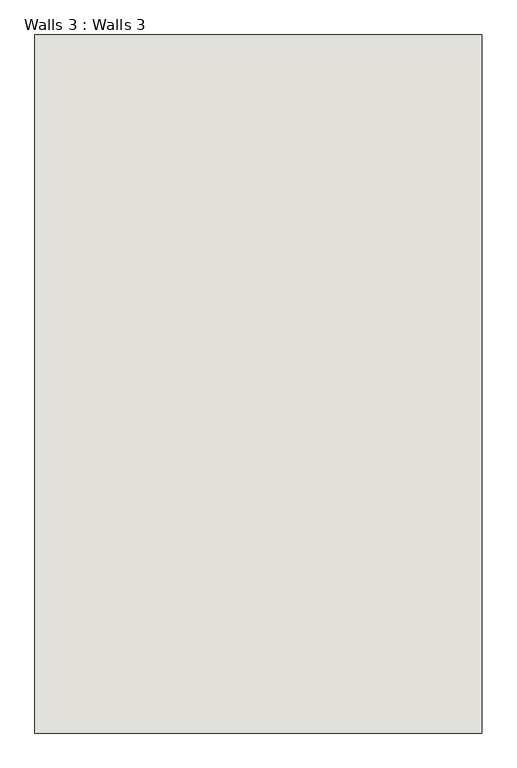
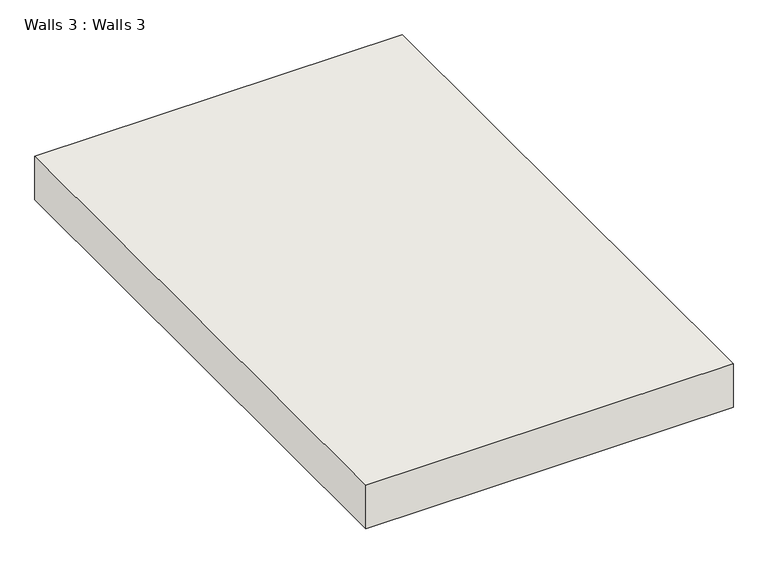
"""IFC4 building model written with IfcOpenShell, lengths in millimetres: wall geometry, Walls 3 : Walls 3."""

from ifc_helpers import new_model, si_unit, frame, origin, place, context, project, spatial, polyline, outline, extrude, source, transform, mapped, element, save


def walls_3_walls_3_115270fa(model_context):
    return source(origin(), model_context, "Body", "SweptSolid", [
        extrude(outline(polyline([(-2632.022521, -16160.3467593), (-8728.022521, -16160.3467593), (-8728.022521, -6638.5230207), (-2632.022521, -6638.5230207), (-2632.022521, -16160.3467593)])), frame((0.0, 0.0, 6096.0), z_axis=(0.0, 0.0, 1.0), x_axis=(1.0, 0.0, 0.0)), (0.0, 0.0, 1.0), 762.0),
    ])


if __name__ == "__main__":
    model = new_model("IFC4")
    model_context = context("Model", 3, world=origin())
    ifc_project = project(units=[si_unit("LENGTHUNIT", "METRE", prefix="MILLI")], contexts=[model_context])
    site = spatial("IfcSite", under=ifc_project)
    building = spatial("IfcBuilding", under=site)
    placement = place(None, origin())
    walls_3_walls_3_shape = walls_3_walls_3_115270fa(model_context)
    element("IfcWall", 1, ObjectType="Walls 3 : Walls 3", at=placement, inside=building, context=model_context, shape_type="MappedRepresentation", body=[
        mapped(walls_3_walls_3_shape, transform((0.0, 0.0, 0.0), x_axis=(1.0, 0.0, 0.0), y_axis=(0.0, 1.0, 0.0), z_axis=(0.0, 0.0, 1.0))),
    ])
    save(model, "model.ifc")

# Revit data of these elements
# Element 1 (IfcWall, "Walls 3 : Walls 3")
#   Materials on its faces: "Default Wall"
# Materials
#   "Default Wall": colour RGB 128 128 128, transparency 0
